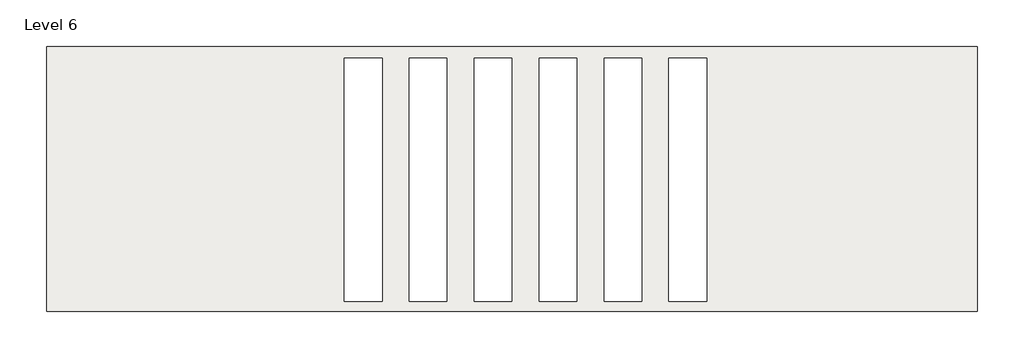
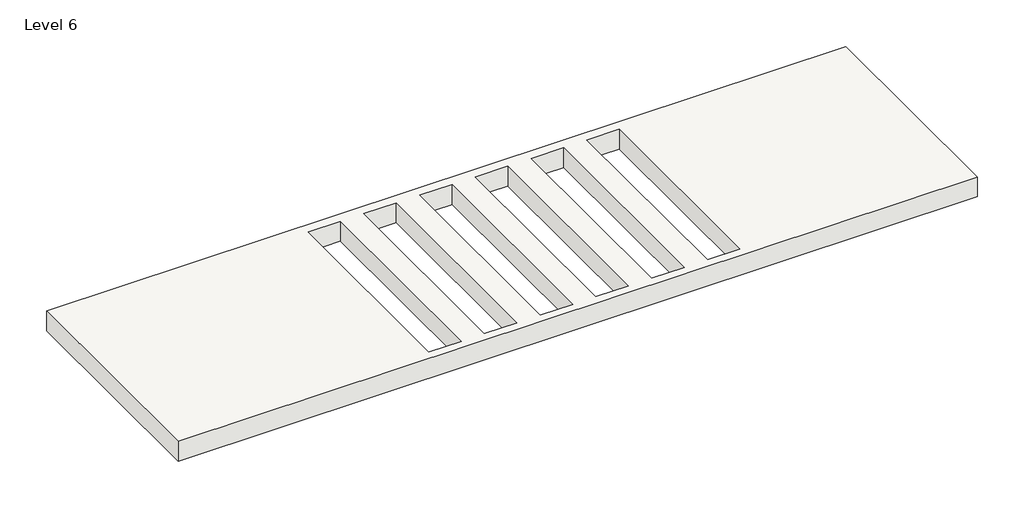
# One storey: 1 roof.
"""IFC4 building model written with IfcOpenShell, lengths in millimetres."""

from ifc_helpers import new_model, si_unit, frame, origin, place, context, project, spatial, polyline, outline, extrude, element, save

model = new_model("IFC4")

# Units and contexts
model_context = context("Model", 3, world=origin())
ifc_project = project(units=[si_unit("LENGTHUNIT", "METRE", prefix="MILLI")], contexts=[model_context])

# Site, building, storey
site = spatial("IfcSite", under=ifc_project)
building = spatial("IfcBuilding", under=site)
storey = spatial("IfcBuildingStorey", under=building, Name="Level 6", Elevation=19202.4)

# Roof
placement = place(None, origin())
element("IfcRoof", 1, ObjectType="Generic - 9\"", at=placement, inside=storey, context=model_context, shape_type="SweptSolid", body=[
    extrude(outline(polyline([(-8833.9561565, 3954.3985991), (-96.3561565, 3954.3985991), (-96.3561565, 1465.1985991), (-8833.9561565, 1465.1985991), (-8833.9561565, 3954.3985991)]), holes=[polyline([(-5685.1030473, 1560.1402851), (-5685.1030473, 3843.629708), (-6039.9561565, 3843.629708), (-6039.9561565, 1560.1402851), (-5685.1030473, 1560.1402851)]), polyline([(-5075.5030473, 1560.1402851), (-5075.5030473, 3843.629708), (-5430.3561565, 3843.629708), (-5430.3561565, 1560.1402851), (-5075.5030473, 1560.1402851)]), polyline([(-4465.9030473, 1560.1402851), (-4465.9030473, 3843.629708), (-4820.7561565, 3843.629708), (-4820.7561565, 1560.1402851), (-4465.9030473, 1560.1402851)]), polyline([(-3856.3030473, 1560.1402851), (-3856.3030473, 3843.629708), (-4211.1561565, 3843.629708), (-4211.1561565, 1560.1402851), (-3856.3030473, 1560.1402851)]), polyline([(-3246.7030473, 1560.1402851), (-3246.7030473, 3843.629708), (-3601.5561565, 3843.629708), (-3601.5561565, 1560.1402851), (-3246.7030473, 1560.1402851)]), polyline([(-2637.1030473, 1560.1402851), (-2637.1030473, 3843.629708), (-2991.9561565, 3843.629708), (-2991.9561565, 1560.1402851), (-2637.1030473, 1560.1402851)])]), frame((0.0, 0.0, 19202.4), z_axis=(0.0, 0.0, 1.0), x_axis=(1.0, 0.0, 0.0)), (0.0, 0.0, 1.0), 228.6),
])

save(model, "model.ifc")

# Revit data of these elements
# Type "Generic - 9\""
#   Assembly Code = "B1020"
#   Layers, outside or top first: 0' - 9" no material (function 1)
# Element 1 (IfcRoof, "Generic - 9\"")
#   built-in parameter 1001705 = 63.75 (stored number, unit not read)
#   built-in parameter 1001710 = 33615
#   Phase Created = New Construction
#   Materials on its faces: "Default Roof"
# Materials
#   "Default Roof": colour RGB 88 101 114, transparency 0
